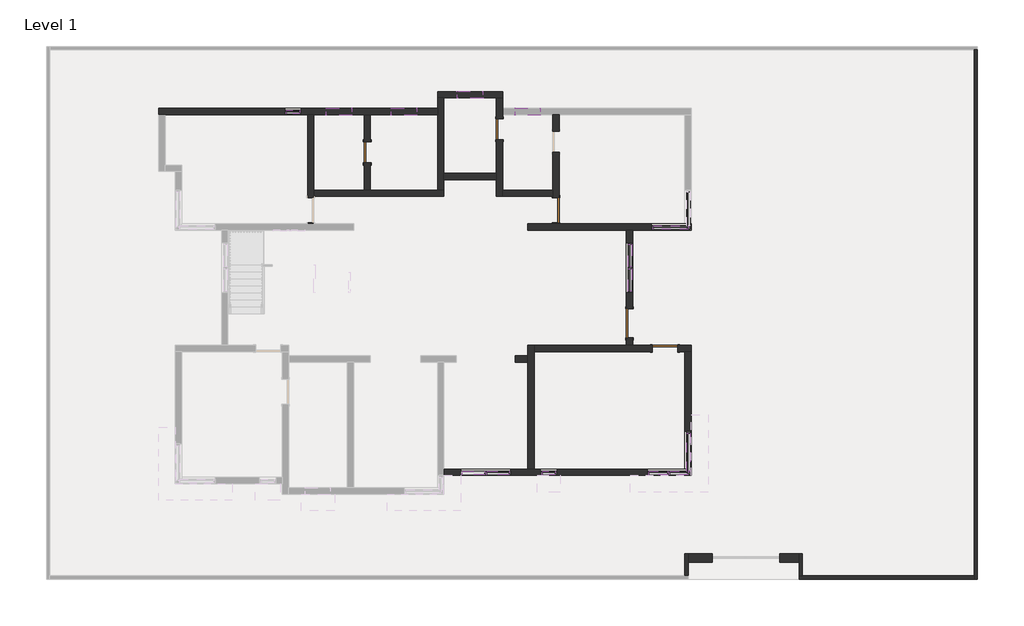
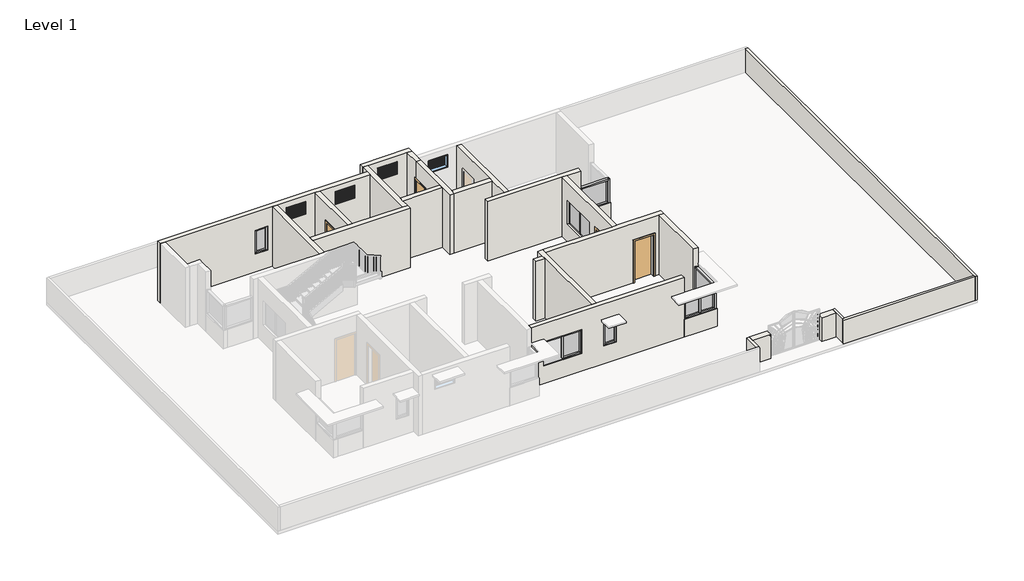
# One storey, part 2 of 9: 37 members, 27 walls, 9 plates, 5 doors, 4 windows.
"""IFC4 building model written with IfcOpenShell, lengths in millimetres."""

from ifc_helpers import new_model, si_unit, frame, origin, origin_with_axes, place, context, project, spatial, polyline, outline, extrude, faceted_brep, transform, mapped, element, save
from components import door_bb98abfd, single_flush_door_3_0ca8825f, door_0848dd25, member_75074519, member_5783932f, member_49503176, member_e1cf819f, member_6e28d7e1, member_2b49869a, member_c17f1be2, member_8d24a278, member_86d06fe4, system_panel_glazed_87944ff9, system_panel_glazed_e0df8542, system_panel_glazed_927b5fc9, system_panel_glazed_d6173012, system_panel_glazed_7cebc396, system_panel_glazed_1bcf12e0, window_a18e4be4

model = new_model("IFC4")

# Units and contexts
model_context = context("Model", 3, world=origin())
ifc_project = project(units=[si_unit("LENGTHUNIT", "METRE", prefix="MILLI")], contexts=[model_context])

# Site, building, storey
site = spatial("IfcSite", under=ifc_project)
building = spatial("IfcBuilding", under=site)
storey = spatial("IfcBuildingStorey", under=building, Name="Level 1", Elevation=0.0)

# Doors
placement = place(None, origin())
door_shape = door_bb98abfd(model_context)
element("IfcDoor", 1, ObjectType="Single-Flush : door 2'6\"", at=placement, inside=storey, context=model_context, shape_type="MappedRepresentation", body=[
    mapped(door_shape, transform((-35934.4146233, 18282.7624892, 0.0), x_axis=(0.0, 1.0, 0.0), y_axis=(-1.0, 0.0, 0.0), z_axis=(0.0, 0.0, 1.0))),
])
element("IfcDoor", 2, ObjectType="Single-Flush : door 2'6\"", at=placement, inside=storey, context=model_context, shape_type="MappedRepresentation", body=[
    mapped(door_shape, transform((-31133.8146233, 19120.9624892, 0.0), x_axis=(0.0, 1.0, 0.0), y_axis=(-1.0, 0.0, 0.0), z_axis=(0.0, 0.0, 1.0))),
])
single_flush_door_3_shape = single_flush_door_3_0ca8825f(model_context)
element("IfcDoor", 3, ObjectType="Single-Flush : door 3'", at=placement, inside=storey, context=model_context, shape_type="MappedRepresentation", body=[
    mapped(single_flush_door_3_shape, transform((-25114.0146233, 11158.0624892, 0.0), x_axis=(1.0, 0.0, 0.0), y_axis=(0.0, 1.0, 0.0), z_axis=(0.0, 0.0, 1.0))),
])
element("IfcDoor", 4, ObjectType="Single-Flush : door 3'", at=placement, inside=storey, context=model_context, shape_type="MappedRepresentation", body=[
    mapped(single_flush_door_3_shape, transform((-29076.4146233, 16187.2624892, 0.0), x_axis=(0.0, -1.0, 0.0), y_axis=(1.0, 0.0, 0.0), z_axis=(0.0, 0.0, 1.0))),
])
door_2_shape = door_0848dd25(model_context)
element("IfcDoor", 5, ObjectType="Single-Flush : door 3'6\"", at=placement, inside=storey, context=model_context, shape_type="MappedRepresentation", body=[
    mapped(door_2_shape, transform((-26409.4146233, 12072.4624892, 0.0), x_axis=(0.0, -1.0, 0.0), y_axis=(1.0, 0.0, 0.0), z_axis=(0.0, 0.0, 1.0))),
])

# Members
member_shape = member_75074519(model_context)
element("IfcMember", 6, ObjectType="Rectangular Mullion : 2.5\" x 5\" rectangular", at=placement, inside=storey, context=model_context, shape_type="MappedRepresentation", body=[
    mapped(member_shape, transform((-24199.6146233, 15552.2624892, 914.4), x_axis=(1.0, 0.0, 0.0), y_axis=(0.0, -1.0, 0.0), z_axis=(0.0, 0.0, -1.0))),
])
element("IfcMember", 7, ObjectType="Rectangular Mullion : 2.5\" x 5\" rectangular", at=placement, inside=storey, context=model_context, shape_type="MappedRepresentation", body=[
    mapped(member_shape, transform((-24199.6146233, 6636.8624892, 914.4), x_axis=(1.0, 0.0, 0.0), y_axis=(0.0, -1.0, 0.0), z_axis=(0.0, 0.0, -1.0))),
])
element("IfcMember", 8, ObjectType="Rectangular Mullion : 2.5\" x 5\" rectangular", at=placement, inside=storey, context=model_context, shape_type="MappedRepresentation", body=[
    mapped(member_shape, transform((-24263.1146233, 8148.1624892, 914.4), x_axis=(0.0, 1.0, 0.0), y_axis=(1.0, 0.0, 0.0), z_axis=(0.0, 0.0, -1.0))),
])
element("IfcMember", 9, ObjectType="Rectangular Mullion : 2.5\" x 5\" rectangular", at=placement, inside=storey, context=model_context, shape_type="MappedRepresentation", body=[
    mapped(member_shape, transform((-30714.7146233, 6636.8624892, 914.4), x_axis=(1.0, 0.0, 0.0), y_axis=(0.0, -1.0, 0.0), z_axis=(0.0, 0.0, -1.0))),
])
element("IfcMember", 10, ObjectType="Rectangular Mullion : 2.5\" x 5\" rectangular", at=placement, inside=storey, context=model_context, shape_type="MappedRepresentation", body=[
    mapped(member_shape, transform((-26383.9055559, 15005.5684528, 914.4), x_axis=(0.0, 1.0, 0.0), y_axis=(1.0, 0.0, 0.0), z_axis=(0.0, 0.0, -1.0))),
])
element("IfcMember", 11, ObjectType="Rectangular Mullion : 2.5\" x 5\" rectangular", at=placement, inside=storey, context=model_context, shape_type="MappedRepresentation", body=[
    mapped(member_shape, transform((-38334.7146233, 19743.2624892, 914.4), x_axis=(1.0, 0.0, 0.0), y_axis=(0.0, -1.0, 0.0), z_axis=(0.0, 0.0, -1.0))),
])
element("IfcMember", 12, ObjectType="Rectangular Mullion : 2.5\" x 5\" rectangular", at=placement, inside=storey, context=model_context, shape_type="MappedRepresentation", body=[
    mapped(member_shape, transform((-29038.3146233, 6636.8624892, 914.4), x_axis=(1.0, 0.0, 0.0), y_axis=(0.0, -1.0, 0.0), z_axis=(0.0, 0.0, -1.0))),
])
element("IfcMember", 13, ObjectType="Rectangular Mullion : 2.5\" x 5\" rectangular", at=placement, inside=storey, context=model_context, shape_type="MappedRepresentation", body=[
    mapped(member_shape, transform((-25609.3146233, 15552.2624892, 2133.6), x_axis=(-1.0, 0.0, 0.0), y_axis=(0.0, -1.0, 0.0), z_axis=(0.0, 0.0, 1.0))),
])
element("IfcMember", 14, ObjectType="Rectangular Mullion : 2.5\" x 5\" rectangular", at=placement, inside=storey, context=model_context, shape_type="MappedRepresentation", body=[
    mapped(member_shape, transform((-24263.1146233, 15552.2624892, 2133.6), x_axis=(0.0, -1.0, 0.0), y_axis=(1.0, 0.0, 0.0), z_axis=(0.0, 0.0, 1.0))),
])
element("IfcMember", 15, ObjectType="Rectangular Mullion : 2.5\" x 5\" rectangular", at=placement, inside=storey, context=model_context, shape_type="MappedRepresentation", body=[
    mapped(member_shape, transform((-25761.7146233, 6636.8624892, 2133.6), x_axis=(-1.0, 0.0, 0.0), y_axis=(0.0, -1.0, 0.0), z_axis=(0.0, 0.0, 1.0))),
])
element("IfcMember", 16, ObjectType="Rectangular Mullion : 2.5\" x 5\" rectangular", at=placement, inside=storey, context=model_context, shape_type="MappedRepresentation", body=[
    mapped(member_shape, transform((-24263.1146233, 6636.8624892, 2133.6), x_axis=(0.0, -1.0, 0.0), y_axis=(1.0, 0.0, 0.0), z_axis=(0.0, 0.0, 1.0))),
])
element("IfcMember", 17, ObjectType="Rectangular Mullion : 2.5\" x 5\" rectangular", at=placement, inside=storey, context=model_context, shape_type="MappedRepresentation", body=[
    mapped(member_shape, transform((-26383.9055559, 13177.3624892, 2133.6), x_axis=(0.0, -1.0, 0.0), y_axis=(1.0, 0.0, 0.0), z_axis=(0.0, 0.0, 1.0))),
])
element("IfcMember", 18, ObjectType="Rectangular Mullion : 2.5\" x 5\" rectangular", at=placement, inside=storey, context=model_context, shape_type="MappedRepresentation", body=[
    mapped(member_shape, transform((-38944.3146233, 19743.2624892, 2133.6), x_axis=(-1.0, 0.0, 0.0), y_axis=(0.0, -1.0, 0.0), z_axis=(0.0, 0.0, 1.0))),
])
element("IfcMember", 19, ObjectType="Rectangular Mullion : 2.5\" x 5\" rectangular", at=placement, inside=storey, context=model_context, shape_type="MappedRepresentation", body=[
    mapped(member_shape, transform((-29647.9146233, 6636.8624892, 2133.6), x_axis=(-1.0, 0.0, 0.0), y_axis=(0.0, -1.0, 0.0), z_axis=(0.0, 0.0, 1.0))),
])
member_2_shape = member_5783932f(model_context)
element("IfcMember", 20, ObjectType="Rectangular Mullion : 2.5\" x 5\" rectangular", at=placement, inside=storey, context=model_context, shape_type="MappedRepresentation", body=[
    mapped(member_2_shape, transform((-24263.1146233, 15552.2624892, 2133.6), x_axis=(0.0, 0.0, 1.0), y_axis=(0.0, -1.0, 0.0), z_axis=(1.0, 0.0, 0.0))),
])
element("IfcMember", 21, ObjectType="Rectangular Mullion : 2.5\" x 5\" rectangular", at=placement, inside=storey, context=model_context, shape_type="MappedRepresentation", body=[
    mapped(member_2_shape, transform((-25545.8146233, 15552.2624892, 914.4), x_axis=(0.0, 0.0, -1.0), y_axis=(0.0, -1.0, 0.0), z_axis=(-1.0, 0.0, 0.0))),
])
member_3_shape = member_49503176(model_context)
element("IfcMember", 22, ObjectType="Rectangular Mullion : 2.5\" x 5\" rectangular", at=placement, inside=storey, context=model_context, shape_type="MappedRepresentation", body=[
    mapped(member_3_shape, transform((-24263.1146233, 15615.7624892, 914.4), x_axis=(0.0, 0.0, -1.0), y_axis=(1.0, 0.0, 0.0), z_axis=(0.0, -1.0, 0.0))),
])
member_4_shape = member_e1cf819f(model_context)
element("IfcMember", 23, ObjectType="Rectangular Mullion : 2.5\" x 5\" rectangular", at=placement, inside=storey, context=model_context, shape_type="MappedRepresentation", body=[
    mapped(member_4_shape, transform((-24263.1146233, 8084.6624892, 2133.6), x_axis=(0.0, 0.0, 1.0), y_axis=(1.0, 0.0, 0.0), z_axis=(0.0, 1.0, 0.0))),
])
element("IfcMember", 24, ObjectType="Rectangular Mullion : 2.5\" x 5\" rectangular", at=placement, inside=storey, context=model_context, shape_type="MappedRepresentation", body=[
    mapped(member_4_shape, transform((-24263.1146233, 6700.3624892, 914.4), x_axis=(0.0, 0.0, -1.0), y_axis=(1.0, 0.0, 0.0), z_axis=(0.0, -1.0, 0.0))),
])
member_5_shape = member_6e28d7e1(model_context)
element("IfcMember", 25, ObjectType="Rectangular Mullion : 2.5\" x 5\" rectangular", at=placement, inside=storey, context=model_context, shape_type="MappedRepresentation", body=[
    mapped(member_5_shape, transform((-24263.1146233, 6636.8624892, 2133.6), x_axis=(0.0, 0.0, 1.0), y_axis=(0.0, -1.0, 0.0), z_axis=(1.0, 0.0, 0.0))),
])
element("IfcMember", 26, ObjectType="Rectangular Mullion : 2.5\" x 5\" rectangular", at=placement, inside=storey, context=model_context, shape_type="MappedRepresentation", body=[
    mapped(member_5_shape, transform((-25012.4146233, 6636.8624892, 2133.6), x_axis=(0.0, 0.0, 1.0), y_axis=(0.0, -1.0, 0.0), z_axis=(1.0, 0.0, 0.0))),
])
element("IfcMember", 27, ObjectType="Rectangular Mullion : 2.5\" x 5\" rectangular", at=placement, inside=storey, context=model_context, shape_type="MappedRepresentation", body=[
    mapped(member_5_shape, transform((-25698.2146233, 6636.8624892, 914.4), x_axis=(0.0, 0.0, -1.0), y_axis=(0.0, -1.0, 0.0), z_axis=(-1.0, 0.0, 0.0))),
])
element("IfcMember", 28, ObjectType="Rectangular Mullion : 2.5\" x 5\" rectangular", at=placement, inside=storey, context=model_context, shape_type="MappedRepresentation", body=[
    mapped(member_5_shape, transform((-24948.9146233, 6636.8624892, 914.4), x_axis=(0.0, 0.0, -1.0), y_axis=(0.0, -1.0, 0.0), z_axis=(-1.0, 0.0, 0.0))),
])
member_6_shape = member_2b49869a(model_context)
element("IfcMember", 29, ObjectType="Rectangular Mullion : 2.5\" x 5\" rectangular", at=placement, inside=storey, context=model_context, shape_type="MappedRepresentation", body=[
    mapped(member_6_shape, transform((-24980.6646233, 6636.8624892, 914.4), x_axis=(1.0, 0.0, 0.0), y_axis=(0.0, -1.0, 0.0), z_axis=(0.0, 0.0, -1.0))),
])
element("IfcMember", 30, ObjectType="Rectangular Mullion : 2.5\" x 5\" rectangular", at=placement, inside=storey, context=model_context, shape_type="MappedRepresentation", body=[
    mapped(member_6_shape, transform((-31629.1146233, 6636.8624892, 914.4), x_axis=(1.0, 0.0, 0.0), y_axis=(0.0, -1.0, 0.0), z_axis=(0.0, 0.0, -1.0))),
])
element("IfcMember", 31, ObjectType="Rectangular Mullion : 2.5\" x 5\" rectangular", at=placement, inside=storey, context=model_context, shape_type="MappedRepresentation", body=[
    mapped(member_6_shape, transform((-26383.9055559, 14091.465471, 914.4), x_axis=(0.0, 1.0, 0.0), y_axis=(1.0, 0.0, 0.0), z_axis=(0.0, 0.0, -1.0))),
])
member_7_shape = member_c17f1be2(model_context)
element("IfcMember", 32, ObjectType="Rectangular Mullion : 2.5\" x 5\" rectangular", at=placement, inside=storey, context=model_context, shape_type="MappedRepresentation", body=[
    mapped(member_7_shape, transform((-30778.2146233, 6636.8624892, 2133.6), x_axis=(0.0, 0.0, 1.0), y_axis=(0.0, -1.0, 0.0), z_axis=(1.0, 0.0, 0.0))),
])
element("IfcMember", 33, ObjectType="Rectangular Mullion : 2.5\" x 5\" rectangular", at=placement, inside=storey, context=model_context, shape_type="MappedRepresentation", body=[
    mapped(member_7_shape, transform((-31660.8646233, 6636.8624892, 2133.6), x_axis=(0.0, 0.0, 1.0), y_axis=(0.0, -1.0, 0.0), z_axis=(1.0, 0.0, 0.0))),
])
element("IfcMember", 34, ObjectType="Rectangular Mullion : 2.5\" x 5\" rectangular", at=placement, inside=storey, context=model_context, shape_type="MappedRepresentation", body=[
    mapped(member_7_shape, transform((-31597.3646233, 6636.8624892, 914.4), x_axis=(0.0, 0.0, -1.0), y_axis=(0.0, -1.0, 0.0), z_axis=(-1.0, 0.0, 0.0))),
])
member_8_shape = member_8d24a278(model_context)
element("IfcMember", 35, ObjectType="Rectangular Mullion : 2.5\" x 5\" rectangular", at=placement, inside=storey, context=model_context, shape_type="MappedRepresentation", body=[
    mapped(member_8_shape, transform((-26383.9055559, 14942.0684528, 2133.6), x_axis=(0.0, 0.0, 1.0), y_axis=(1.0, 0.0, 0.0), z_axis=(0.0, 1.0, 0.0))),
])
element("IfcMember", 36, ObjectType="Rectangular Mullion : 2.5\" x 5\" rectangular", at=placement, inside=storey, context=model_context, shape_type="MappedRepresentation", body=[
    mapped(member_8_shape, transform((-26383.9055559, 14059.715471, 2133.6), x_axis=(0.0, 0.0, 1.0), y_axis=(1.0, 0.0, 0.0), z_axis=(0.0, 1.0, 0.0))),
])
element("IfcMember", 37, ObjectType="Rectangular Mullion : 2.5\" x 5\" rectangular", at=placement, inside=storey, context=model_context, shape_type="MappedRepresentation", body=[
    mapped(member_8_shape, transform((-26383.9055559, 13240.8624892, 914.4), x_axis=(0.0, 0.0, -1.0), y_axis=(1.0, 0.0, 0.0), z_axis=(0.0, -1.0, 0.0))),
])
element("IfcMember", 38, ObjectType="Rectangular Mullion : 2.5\" x 5\" rectangular", at=placement, inside=storey, context=model_context, shape_type="MappedRepresentation", body=[
    mapped(member_8_shape, transform((-26383.9055559, 14123.215471, 914.4), x_axis=(0.0, 0.0, -1.0), y_axis=(1.0, 0.0, 0.0), z_axis=(0.0, -1.0, 0.0))),
])
member_9_shape = member_86d06fe4(model_context)
element("IfcMember", 39, ObjectType="Rectangular Mullion : 2.5\" x 5\" rectangular", at=placement, inside=storey, context=model_context, shape_type="MappedRepresentation", body=[
    mapped(member_9_shape, transform((-38398.2146233, 19743.2624892, 2133.6), x_axis=(0.0, 0.0, 1.0), y_axis=(0.0, -1.0, 0.0), z_axis=(1.0, 0.0, 0.0))),
])
element("IfcMember", 40, ObjectType="Rectangular Mullion : 2.5\" x 5\" rectangular", at=placement, inside=storey, context=model_context, shape_type="MappedRepresentation", body=[
    mapped(member_9_shape, transform((-29101.8146233, 6636.8624892, 2133.6), x_axis=(0.0, 0.0, 1.0), y_axis=(0.0, -1.0, 0.0), z_axis=(1.0, 0.0, 0.0))),
])
element("IfcMember", 41, ObjectType="Rectangular Mullion : 2.5\" x 5\" rectangular", at=placement, inside=storey, context=model_context, shape_type="MappedRepresentation", body=[
    mapped(member_9_shape, transform((-38880.8146233, 19743.2624892, 914.4), x_axis=(0.0, 0.0, -1.0), y_axis=(0.0, -1.0, 0.0), z_axis=(-1.0, 0.0, 0.0))),
])
element("IfcMember", 42, ObjectType="Rectangular Mullion : 2.5\" x 5\" rectangular", at=placement, inside=storey, context=model_context, shape_type="MappedRepresentation", body=[
    mapped(member_9_shape, transform((-29584.4146233, 6636.8624892, 914.4), x_axis=(0.0, 0.0, -1.0), y_axis=(0.0, -1.0, 0.0), z_axis=(-1.0, 0.0, 0.0))),
])

# Plates
system_panel_glazed_shape = system_panel_glazed_87944ff9(model_context)
element("IfcPlate", 43, ObjectType="System Panel : Glazed", at=placement, inside=storey, context=model_context, shape_type="MappedRepresentation", body=[
    mapped(system_panel_glazed_shape, transform((-24904.4646233, 15552.2624892, 977.9), x_axis=(1.0, 0.0, 0.0), y_axis=(0.0, 1.0, 0.0), z_axis=(0.0, 0.0, 1.0))),
])
system_panel_glazed_2_shape = system_panel_glazed_e0df8542(model_context)
element("IfcPlate", 44, ObjectType="System Panel : Glazed", at=placement, inside=storey, context=model_context, shape_type="MappedRepresentation", body=[
    mapped(system_panel_glazed_2_shape, transform((-24263.1146233, 7392.5124892, 977.9), x_axis=(0.0, 1.0, 0.0), y_axis=(-1.0, 0.0, 0.0), z_axis=(0.0, 0.0, 1.0))),
])
system_panel_glazed_3_shape = system_panel_glazed_927b5fc9(model_context)
element("IfcPlate", 45, ObjectType="System Panel : Glazed", at=placement, inside=storey, context=model_context, shape_type="MappedRepresentation", body=[
    mapped(system_panel_glazed_3_shape, transform((-25355.3146233, 6636.8624892, 977.9), x_axis=(1.0, 0.0, 0.0), y_axis=(0.0, 1.0, 0.0), z_axis=(0.0, 0.0, 1.0))),
])
element("IfcPlate", 46, ObjectType="System Panel : Glazed", at=placement, inside=storey, context=model_context, shape_type="MappedRepresentation", body=[
    mapped(system_panel_glazed_3_shape, transform((-24606.0146233, 6636.8624892, 977.9), x_axis=(1.0, 0.0, 0.0), y_axis=(0.0, 1.0, 0.0), z_axis=(0.0, 0.0, 1.0))),
])
system_panel_glazed_4_shape = system_panel_glazed_d6173012(model_context)
element("IfcPlate", 47, ObjectType="System Panel : Glazed", at=placement, inside=storey, context=model_context, shape_type="MappedRepresentation", body=[
    mapped(system_panel_glazed_4_shape, transform((-31187.7896233, 6636.8624892, 977.9), x_axis=(1.0, 0.0, 0.0), y_axis=(0.0, 1.0, 0.0), z_axis=(0.0, 0.0, 1.0))),
])
system_panel_glazed_5_shape = system_panel_glazed_7cebc396(model_context)
element("IfcPlate", 48, ObjectType="System Panel : Glazed", at=placement, inside=storey, context=model_context, shape_type="MappedRepresentation", body=[
    mapped(system_panel_glazed_5_shape, transform((-26383.9055559, 13650.2889801, 977.9), x_axis=(0.0, 1.0, 0.0), y_axis=(-1.0, 0.0, 0.0), z_axis=(0.0, 0.0, 1.0))),
])
element("IfcPlate", 49, ObjectType="System Panel : Glazed", at=placement, inside=storey, context=model_context, shape_type="MappedRepresentation", body=[
    mapped(system_panel_glazed_5_shape, transform((-26383.9055559, 14532.6419619, 977.9), x_axis=(0.0, 1.0, 0.0), y_axis=(-1.0, 0.0, 0.0), z_axis=(0.0, 0.0, 1.0))),
])
system_panel_glazed_6_shape = system_panel_glazed_1bcf12e0(model_context)
element("IfcPlate", 50, ObjectType="System Panel : Glazed", at=placement, inside=storey, context=model_context, shape_type="MappedRepresentation", body=[
    mapped(system_panel_glazed_6_shape, transform((-38639.5146233, 19743.2624892, 977.9), x_axis=(1.0, 0.0, 0.0), y_axis=(0.0, 1.0, 0.0), z_axis=(0.0, 0.0, 1.0))),
])
element("IfcPlate", 51, ObjectType="System Panel : Glazed", at=placement, inside=storey, context=model_context, shape_type="MappedRepresentation", body=[
    mapped(system_panel_glazed_6_shape, transform((-29343.1146233, 6636.8624892, 977.9), x_axis=(1.0, 0.0, 0.0), y_axis=(0.0, 1.0, 0.0), z_axis=(0.0, 0.0, 1.0))),
])

# Walls
element("IfcWall", 52, at=placement, inside=storey, context=model_context, shape_type="Brep", body=[
    faceted_brep([(-13874.5146233, 22016.5624892, 0.0), (-13874.5146233, 2890.3624892, 0.0), (-13874.5146233, 2776.0624892, 0.0), (-13874.5146233, 2776.0624892, 1219.2), (-13874.5146233, 2890.3624892, 1219.2), (-13874.5146233, 22016.5624892, 1219.2), (-13760.2146233, 22016.5624892, 0.0), (-13760.2146233, 22016.5624892, 1219.2), (-13760.2146233, 2776.0624892, 1219.2), (-13760.2146233, 2776.0624892, 0.0)], [[[0, 1, 2, 3, 4, 5]], [[6, 7, 8, 9]], [[2, 1, 0, 6, 9]], [[5, 4, 3, 8, 7]], [[0, 5, 7, 6]], [[3, 2, 9, 8]]]),
])
element("IfcWall", 53, at=placement, inside=storey, context=model_context, shape_type="Brep", body=[
    faceted_brep([(-13874.5146233, 2890.3624892, 0.0), (-20122.9146233, 2890.3624892, 0.0), (-20237.2146233, 2890.3624892, 0.0), (-20237.2146233, 2890.3624892, 1219.2), (-20122.9146233, 2890.3624892, 1219.2), (-13874.5146233, 2890.3624892, 1219.2), (-13874.5146233, 2776.0624892, 0.0), (-13874.5146233, 2776.0624892, 1219.2), (-20237.2146233, 2776.0624892, 1219.2), (-20237.2146233, 2776.0624892, 0.0)], [[[0, 1, 2, 3, 4, 5]], [[6, 7, 8, 9]], [[2, 1, 0, 6, 9]], [[5, 4, 3, 8, 7]], [[0, 5, 7, 6]], [[3, 2, 9, 8]]]),
])
element("IfcWall", 54, at=placement, inside=storey, context=model_context, shape_type="Brep", body=[
    faceted_brep([(-20122.9146233, 2890.3624892, 0.0), (-20122.9146233, 3690.4624892, 0.0), (-20122.9146233, 3690.4624892, 1219.2), (-20122.9146233, 2890.3624892, 1219.2), (-20237.2146233, 2890.3624892, 0.0), (-20237.2146233, 2890.3624892, 1219.2), (-20237.2146233, 3385.6624892, 1219.2), (-20237.2146233, 3690.4624892, 1219.2), (-20237.2146233, 3690.4624892, 0.0), (-20237.2146233, 3385.6624892, 0.0)], [[[0, 1, 2, 3]], [[4, 5, 6, 7, 8, 9]], [[1, 0, 4, 9, 8]], [[3, 2, 7, 6, 5]], [[0, 3, 5, 4]], [[2, 1, 8, 7]]]),
])
element("IfcWall", 55, at=placement, inside=storey, context=model_context, shape_type="Brep", body=[
    faceted_brep([(-24275.8146233, 2890.3624892, 0.0), (-24275.8146233, 3385.6624892, 0.0), (-24275.8146233, 3690.4624892, 0.0), (-24275.8146233, 3690.4624892, 1219.2), (-24275.8146233, 3385.6624892, 1219.2), (-24275.8146233, 2890.3624892, 1219.2), (-24390.1146233, 2890.3624892, 0.0), (-24390.1146233, 2890.3624892, 1219.2), (-24390.1146233, 3690.4624892, 1219.2), (-24390.1146233, 3690.4624892, 0.0)], [[[0, 1, 2, 3, 4, 5]], [[6, 7, 8, 9]], [[2, 1, 0, 6, 9]], [[5, 4, 3, 8, 7]], [[0, 5, 7, 6]], [[3, 2, 9, 8]]]),
])
element("IfcWall", 56, ObjectType="WALL 9\"", at=placement, inside=storey, context=model_context, shape_type="Brep", body=[
    faceted_brep([(-43516.3146233, 19654.3624892, 0.0), (-43287.7146233, 19654.3624892, 0.0), (-38106.1146233, 19654.3624892, 0.0), (-37877.5146233, 19654.3624892, 0.0), (-36048.7146233, 19654.3624892, 0.0), (-35820.1146233, 19654.3624892, 0.0), (-33381.7146233, 19654.3624892, 0.0), (-33381.7146233, 19654.3624892, 3048.0), (-35820.1146233, 19654.3624892, 3048.0), (-36048.7146233, 19654.3624892, 3048.0), (-37877.5146233, 19654.3624892, 3048.0), (-38106.1146233, 19654.3624892, 3048.0), (-43287.7146233, 19654.3624892, 3048.0), (-43516.3146233, 19654.3624892, 3048.0), (-38944.3146233, 19654.3624892, 914.4), (-38944.3146233, 19654.3624892, 2133.6), (-38334.7146233, 19654.3624892, 2133.6), (-38334.7146233, 19654.3624892, 914.4), (-36505.9146233, 19654.3624892, 2743.2), (-36505.9146233, 19654.3624892, 2133.6), (-37420.3146233, 19654.3624892, 2133.6), (-37420.3146233, 19654.3624892, 2743.2), (-34143.7146233, 19654.3624892, 2743.2), (-34143.7146233, 19654.3624892, 2133.6), (-35058.1146233, 19654.3624892, 2133.6), (-35058.1146233, 19654.3624892, 2743.2), (-33381.7146233, 19882.9624892, 0.0), (-43516.3146233, 19882.9624892, 0.0), (-43516.3146233, 19882.9624892, 3048.0), (-33381.7146233, 19882.9624892, 3048.0), (-38944.3146233, 19882.9624892, 2133.6), (-38944.3146233, 19882.9624892, 914.4), (-38334.7146233, 19882.9624892, 914.4), (-38334.7146233, 19882.9624892, 2133.6), (-36505.9146233, 19882.9624892, 2743.2), (-37420.3146233, 19882.9624892, 2743.2), (-37420.3146233, 19882.9624892, 2133.6), (-36505.9146233, 19882.9624892, 2133.6), (-34143.7146233, 19882.9624892, 2743.2), (-35058.1146233, 19882.9624892, 2743.2), (-35058.1146233, 19882.9624892, 2133.6), (-34143.7146233, 19882.9624892, 2133.6)], [[[0, 1, 2, 3, 4, 5, 6, 7, 8, 9, 10, 11, 12, 13], [14, 15, 16, 17], [18, 19, 20, 21], [22, 23, 24, 25]], [[26, 27, 28, 29], [30, 31, 32, 33], [34, 35, 36, 37], [38, 39, 40, 41]], [[6, 5, 4, 3, 2, 1, 0, 27, 26]], [[13, 12, 11, 10, 9, 8, 7, 29, 28]], [[0, 13, 28, 27]], [[7, 6, 26, 29]], [[14, 31, 30, 15]], [[15, 30, 33, 16]], [[16, 33, 32, 17]], [[31, 14, 17, 32]], [[19, 18, 34, 37]], [[20, 19, 37, 36]], [[21, 20, 36, 35]], [[18, 21, 35, 34]], [[23, 22, 38, 41]], [[24, 23, 41, 40]], [[25, 24, 40, 39]], [[22, 25, 39, 38]]]),
])
element("IfcWall", 57, ObjectType="WALL 9\"", at=placement, inside=storey, context=model_context, shape_type="Brep", body=[
    faceted_brep([(-33381.7146233, 20263.9624892, 0.0), (-33153.1146233, 20263.9624892, 0.0), (-31248.1146233, 20263.9624892, 0.0), (-31019.5146233, 20263.9624892, 0.0), (-31019.5146233, 20263.9624892, 3048.0), (-31248.1146233, 20263.9624892, 3048.0), (-33153.1146233, 20263.9624892, 3048.0), (-33381.7146233, 20263.9624892, 3048.0), (-31743.4146233, 20263.9624892, 2743.2), (-31743.4146233, 20263.9624892, 2133.6), (-32657.8146233, 20263.9624892, 2133.6), (-32657.8146233, 20263.9624892, 2743.2), (-33381.7146233, 20492.5624892, 0.0), (-33381.7146233, 20492.5624892, 3048.0), (-31019.5146233, 20492.5624892, 3048.0), (-31019.5146233, 20492.5624892, 0.0), (-31743.4146233, 20492.5624892, 2743.2), (-32657.8146233, 20492.5624892, 2743.2), (-32657.8146233, 20492.5624892, 2133.6), (-31743.4146233, 20492.5624892, 2133.6)], [[[0, 1, 2, 3, 4, 5, 6, 7], [8, 9, 10, 11]], [[12, 13, 14, 15], [16, 17, 18, 19]], [[3, 2, 1, 0, 12, 15]], [[7, 6, 5, 4, 14, 13]], [[4, 3, 15, 14]], [[0, 7, 13, 12]], [[9, 8, 16, 19]], [[10, 9, 19, 18]], [[11, 10, 18, 17]], [[8, 11, 17, 16]]]),
])
element("IfcWall", 58, ObjectType="WALL 9\"", at=placement, inside=storey, context=model_context, shape_type="Brep", body=[
    faceted_brep([(-31248.1146233, 20263.9624892, 0.0), (-31248.1146233, 19501.9624892, 0.0), (-31248.1146233, 19501.9624892, 2133.6), (-31248.1146233, 19501.9624892, 3048.0), (-31248.1146233, 20263.9624892, 3048.0), (-31019.5146233, 20263.9624892, 0.0), (-31019.5146233, 20263.9624892, 3048.0), (-31019.5146233, 19882.9624892, 3048.0), (-31019.5146233, 19654.3624892, 3048.0), (-31019.5146233, 19501.9624892, 3048.0), (-31019.5146233, 19501.9624892, 2133.6), (-31019.5146233, 19501.9624892, 0.0), (-31019.5146233, 19654.3624892, 0.0), (-31019.5146233, 19882.9624892, 0.0)], [[[0, 1, 2, 3, 4]], [[5, 6, 7, 8, 9, 10, 11, 12, 13]], [[1, 0, 5, 13, 12, 11]], [[3, 2, 1, 11, 10, 9]], [[4, 3, 9, 8, 7, 6]], [[0, 4, 6, 5]]]),
])
element("IfcWall", 59, ObjectType="WALL 9\" 2", at=placement, inside=storey, context=model_context, shape_type="Brep", body=[
    faceted_brep([(-33152.7428374, 6547.9624892, 0.0), (-25761.7146233, 6547.9624892, 0.0), (-25761.7146233, 6547.9624892, 914.4), (-25761.7146233, 6547.9624892, 2133.6), (-25761.7146233, 6547.9624892, 3048.0), (-33152.7428374, 6547.9624892, 3048.0), (-32543.5146233, 6547.9624892, 914.4), (-32543.5146233, 6547.9624892, 2133.6), (-30714.7146233, 6547.9624892, 2133.6), (-30714.7146233, 6547.9624892, 914.4), (-29647.9146233, 6547.9624892, 914.4), (-29647.9146233, 6547.9624892, 2133.6), (-29038.3146233, 6547.9624892, 2133.6), (-29038.3146233, 6547.9624892, 914.4), (-25761.7146233, 6776.5624892, 0.0), (-29876.5146233, 6776.5624892, 0.0), (-30105.1146233, 6776.5624892, 0.0), (-33152.7428374, 6776.5624892, 0.0), (-33152.7428374, 6776.5624892, 3048.0), (-30105.1146233, 6776.5624892, 3048.0), (-29876.5146233, 6776.5624892, 3048.0), (-25761.7146233, 6776.5624892, 3048.0), (-25761.7146233, 6776.5624892, 2133.6), (-25761.7146233, 6776.5624892, 914.4), (-32543.5146233, 6776.5624892, 2133.6), (-32543.5146233, 6776.5624892, 914.4), (-30714.7146233, 6776.5624892, 914.4), (-30714.7146233, 6776.5624892, 2133.6), (-29647.9146233, 6776.5624892, 2133.6), (-29647.9146233, 6776.5624892, 914.4), (-29038.3146233, 6776.5624892, 914.4), (-29038.3146233, 6776.5624892, 2133.6)], [[[0, 1, 2, 3, 4, 5], [6, 7, 8, 9], [10, 11, 12, 13]], [[14, 15, 16, 17, 18, 19, 20, 21, 22, 23], [24, 25, 26, 27], [28, 29, 30, 31]], [[1, 0, 17, 16, 15, 14]], [[5, 4, 21, 20, 19, 18]], [[5, 18, 17, 0]], [[1, 14, 23, 22, 21, 4, 3, 2]], [[6, 25, 24, 7]], [[7, 24, 27, 8]], [[8, 27, 26, 9]], [[25, 6, 9, 26]], [[10, 29, 28, 11]], [[11, 28, 31, 12]], [[12, 31, 30, 13]], [[29, 10, 13, 30]]]),
])
element("IfcWall", 60, ObjectType="WALL 9\" 2", at=placement, inside=storey, context=model_context, shape_type="Brep", body=[
    faceted_brep([(-29876.5146233, 6776.5624892, 0.0), (-29876.5146233, 11043.7624892, 0.0), (-29876.5146233, 11272.3624892, 0.0), (-29876.5146233, 11272.3624892, 3048.0), (-29876.5146233, 11043.7624892, 3048.0), (-29876.5146233, 6776.5624892, 3048.0), (-30105.1146233, 6776.5624892, 0.0), (-30105.1146233, 6776.5624892, 3048.0), (-30105.1146233, 10662.7624892, 3048.0), (-30105.1146233, 10891.3624892, 3048.0), (-30105.1146233, 11272.3624892, 3048.0), (-30105.1146233, 11272.3624892, 0.0), (-30105.1146233, 10891.3624892, 0.0), (-30105.1146233, 10662.7624892, 0.0)], [[[0, 1, 2, 3, 4, 5]], [[6, 7, 8, 9, 10, 11, 12, 13]], [[2, 1, 0, 6, 13, 12, 11]], [[5, 4, 3, 10, 9, 8, 7]], [[0, 5, 7, 6]], [[3, 2, 11, 10]]]),
])
element("IfcWall", 61, ObjectType="WALL 9\" 2", at=placement, inside=storey, context=model_context, shape_type="Brep", body=[
    faceted_brep([(-24656.8146233, 11043.7624892, 2133.6), (-24656.8146233, 11043.7624892, 0.0), (-24390.1146233, 11043.7624892, 0.0), (-24161.5146233, 11043.7624892, 0.0), (-24161.5146233, 11043.7624892, 3048.0), (-24390.1146233, 11043.7624892, 3048.0), (-29876.5146233, 11043.7624892, 3048.0), (-29876.5146233, 11043.7624892, 0.0), (-25571.2146233, 11043.7624892, 0.0), (-25571.2146233, 11043.7624892, 2133.6), (-24161.5146233, 11272.3624892, 0.0), (-24656.8146233, 11272.3624892, 0.0), (-24656.8146233, 11272.3624892, 2133.6), (-25571.2146233, 11272.3624892, 2133.6), (-25571.2146233, 11272.3624892, 0.0), (-26295.1146233, 11272.3624892, 0.0), (-26523.7146233, 11272.3624892, 0.0), (-29876.5146233, 11272.3624892, 0.0), (-29876.5146233, 11272.3624892, 3048.0), (-26523.7146233, 11272.3624892, 3048.0), (-26295.1146233, 11272.3624892, 3048.0), (-24161.5146233, 11272.3624892, 3048.0)], [[[0, 1, 2, 3, 4, 5, 6, 7, 8, 9]], [[10, 11, 12, 13, 14, 15, 16, 17, 18, 19, 20, 21]], [[8, 7, 17, 16, 15, 14]], [[3, 2, 1, 11, 10]], [[6, 5, 4, 21, 20, 19, 18]], [[7, 6, 18, 17]], [[4, 3, 10, 21]], [[12, 11, 1, 0]], [[13, 12, 0, 9]], [[14, 13, 9, 8]]]),
])
element("IfcWall", 62, ObjectType="WALL 9\" 2", at=placement, inside=storey, context=model_context, shape_type="Brep", body=[
    faceted_brep([(-24390.1146233, 11043.7624892, 0.0), (-24390.1146233, 8148.1624892, 0.0), (-24390.1146233, 8148.1624892, 914.4), (-24390.1146233, 8148.1624892, 2133.6), (-24390.1146233, 8148.1624892, 3048.0), (-24390.1146233, 11043.7624892, 3048.0), (-24161.5146233, 11043.7624892, 0.0), (-24161.5146233, 11043.7624892, 3048.0), (-24161.5146233, 8148.1624892, 3048.0), (-24161.5146233, 8148.1624892, 2133.6), (-24161.5146233, 8148.1624892, 914.4), (-24161.5146233, 8148.1624892, 0.0)], [[[0, 1, 2, 3, 4, 5]], [[6, 7, 8, 9, 10, 11]], [[1, 0, 6, 11]], [[5, 4, 8, 7]], [[0, 5, 7, 6]], [[1, 11, 10, 9, 8, 4, 3, 2]]]),
])
element("IfcWall", 63, ObjectType="WALL 9\" 2", at=placement, inside=storey, context=model_context, shape_type="SweptSolid", body=[
    extrude(outline(polyline([(11539.0624892, 2133.6), (11539.0624892, 0.0), (11272.3624892, 0.0), (11272.3624892, 3048.0), (15463.3624892, 3048.0), (15463.3624892, 0.0), (12605.8624892, 0.0), (12605.8624892, 2133.6), (11539.0624892, 2133.6)]), holes=[polyline([(13177.3624892, 2133.6), (13177.3624892, 914.4), (15005.5684528, 914.4), (15005.5684528, 2133.6), (13177.3624892, 2133.6)])]), frame((-26523.7146233, 0.0, 0.0), z_axis=(1.0, 0.0, 0.0), x_axis=(0.0, 1.0, 0.0)), (0.0, 0.0, 1.0), 228.6),
])
element("IfcWall", 64, ObjectType="WALL 9\" 2", at=placement, inside=storey, context=model_context, shape_type="Brep", body=[
    faceted_brep([(-30105.1146233, 15463.3624892, 0.0), (-26523.7146233, 15463.3624892, 0.0), (-26295.1146233, 15463.3624892, 0.0), (-25609.3146233, 15463.3624892, 0.0), (-25609.3146233, 15463.3624892, 914.4), (-25609.3146233, 15463.3624892, 2133.6), (-25609.3146233, 15463.3624892, 3048.0), (-26295.1146233, 15463.3624892, 3048.0), (-26523.7146233, 15463.3624892, 3048.0), (-30105.1146233, 15463.3624892, 3048.0), (-30105.1146233, 15691.9624892, 0.0), (-30105.1146233, 15691.9624892, 3048.0), (-29190.7146233, 15691.9624892, 3048.0), (-28962.1146233, 15691.9624892, 3048.0), (-25609.3146233, 15691.9624892, 3048.0), (-25609.3146233, 15691.9624892, 2133.6), (-25609.3146233, 15691.9624892, 914.4), (-25609.3146233, 15691.9624892, 0.0), (-28962.1146233, 15691.9624892, 0.0), (-29190.7146233, 15691.9624892, 0.0)], [[[0, 1, 2, 3, 4, 5, 6, 7, 8, 9]], [[10, 11, 12, 13, 14, 15, 16, 17, 18, 19]], [[3, 2, 1, 0, 10, 19, 18, 17]], [[9, 8, 7, 6, 14, 13, 12, 11]], [[0, 9, 11, 10]], [[3, 17, 16, 15, 14, 6, 5, 4]]]),
])
element("IfcWall", 65, ObjectType="WALL 9\" 2", at=placement, inside=storey, context=model_context, shape_type="Brep", body=[
    faceted_brep([(-38106.1146233, 15725.5641869, 2133.6), (-38106.1146233, 15725.5641869, 0.0), (-38106.1146233, 15682.9658846, 0.0), (-38106.1146233, 15682.9658846, 3048.0), (-38106.1146233, 19654.3624892, 3048.0), (-38106.1146233, 19654.3624892, 0.0), (-38106.1146233, 16639.9641869, 0.0), (-38106.1146233, 16639.9641869, 2133.6), (-37877.5146233, 15682.9658846, 0.0), (-37877.5146233, 15725.5641869, 0.0), (-37877.5146233, 15725.5641869, 2133.6), (-37877.5146233, 16639.9641869, 2133.6), (-37877.5146233, 16639.9641869, 0.0), (-37877.5146233, 16682.5624892, 0.0), (-37877.5146233, 16911.1624892, 0.0), (-37877.5146233, 19654.3624892, 0.0), (-37877.5146233, 19654.3624892, 3048.0), (-37877.5146233, 16911.1624892, 3048.0), (-37877.5146233, 16682.5624892, 3048.0), (-37877.5146233, 15682.9658846, 3048.0)], [[[0, 1, 2, 3, 4, 5, 6, 7]], [[8, 9, 10, 11, 12, 13, 14, 15, 16, 17, 18, 19]], [[6, 5, 15, 14, 13, 12]], [[2, 1, 9, 8]], [[4, 3, 19, 18, 17, 16]], [[5, 4, 16, 15]], [[3, 2, 8, 19]], [[10, 9, 1, 0]], [[11, 10, 0, 7]], [[12, 11, 7, 6]]]),
])
element("IfcWall", 66, ObjectType="WALL 9\" 2", at=placement, inside=storey, context=model_context, shape_type="Brep", body=[
    faceted_brep([(-37877.5146233, 16682.5624892, 0.0), (-33153.1146233, 16682.5624892, 0.0), (-33153.1146233, 16682.5624892, 3048.0), (-37877.5146233, 16682.5624892, 3048.0), (-37877.5146233, 16911.1624892, 0.0), (-37877.5146233, 16911.1624892, 3048.0), (-36048.7146233, 16911.1624892, 3048.0), (-35820.1146233, 16911.1624892, 3048.0), (-33381.7146233, 16911.1624892, 3048.0), (-33153.1146233, 16911.1624892, 3048.0), (-33153.1146233, 16911.1624892, 0.0), (-33381.7146233, 16911.1624892, 0.0), (-35820.1146233, 16911.1624892, 0.0), (-36048.7146233, 16911.1624892, 0.0)], [[[0, 1, 2, 3]], [[4, 5, 6, 7, 8, 9, 10, 11, 12, 13]], [[1, 0, 4, 13, 12, 11, 10]], [[3, 2, 9, 8, 7, 6, 5]], [[2, 1, 10, 9]], [[0, 3, 5, 4]]]),
])
element("IfcWall", 67, ObjectType="WALL 9\" 2", at=placement, inside=storey, context=model_context, shape_type="SweptSolid", body=[
    extrude(outline(polyline([(19654.3624892, 0.0), (18663.7624892, 0.0), (18663.7624892, 2133.6), (17901.7624892, 2133.6), (17901.7624892, 0.0), (16911.1624892, 0.0), (16911.1624892, 3048.0), (19654.3624892, 3048.0), (19654.3624892, 0.0)])), frame((-36048.7146233, 0.0, 0.0), z_axis=(1.0, 0.0, 0.0), x_axis=(0.0, 1.0, 0.0)), (0.0, 0.0, 1.0), 228.6),
])
element("IfcWall", 68, ObjectType="WALL 9\" 2", at=placement, inside=storey, context=model_context, shape_type="Brep", body=[
    faceted_brep([(-33153.1146233, 16911.1624892, 0.0), (-33153.1146233, 17292.1624892, 0.0), (-33153.1146233, 17520.7624892, 0.0), (-33153.1146233, 20263.9624892, 0.0), (-33153.1146233, 20263.9624892, 3048.0), (-33153.1146233, 17520.7624892, 3048.0), (-33153.1146233, 17292.1624892, 3048.0), (-33153.1146233, 16911.1624892, 3048.0), (-33381.7146233, 16911.1624892, 0.0), (-33381.7146233, 16911.1624892, 3048.0), (-33381.7146233, 19654.3624892, 3048.0), (-33381.7146233, 19882.9624892, 3048.0), (-33381.7146233, 20263.9624892, 3048.0), (-33381.7146233, 20263.9624892, 0.0), (-33381.7146233, 19882.9624892, 0.0), (-33381.7146233, 19654.3624892, 0.0)], [[[0, 1, 2, 3, 4, 5, 6, 7]], [[8, 9, 10, 11, 12, 13, 14, 15]], [[3, 2, 1, 0, 8, 15, 14, 13]], [[7, 6, 5, 4, 12, 11, 10, 9]], [[4, 3, 13, 12]], [[0, 7, 9, 8]]]),
])
element("IfcWall", 69, ObjectType="WALL 9\" 2", at=placement, inside=storey, context=model_context, shape_type="SweptSolid", body=[
    extrude(outline(polyline([(-31248.1146233, 17292.1624892), (-33153.1146233, 17292.1624892), (-33153.1146233, 17520.7624892), (-31248.1146233, 17520.7624892), (-31248.1146233, 17292.1624892)])), origin_with_axes(), (0.0, 0.0, 1.0), 3048.0),
])
element("IfcWall", 70, ObjectType="WALL 9\" 2", at=placement, inside=storey, context=model_context, shape_type="Brep", body=[
    faceted_brep([(-31248.1146233, 16682.5624892, 3048.0), (-31248.1146233, 17292.1624892, 3048.0), (-31248.1146233, 17520.7624892, 3048.0), (-31248.1146233, 19501.9624892, 3048.0), (-31248.1146233, 19501.9624892, 2133.6), (-31248.1146233, 18739.9624892, 2133.6), (-31248.1146233, 18739.9624892, 0.0), (-31248.1146233, 17520.7624892, 0.0), (-31248.1146233, 17292.1624892, 0.0), (-31248.1146233, 16682.5624892, 0.0), (-31019.5146233, 19501.9624892, 3048.0), (-31019.5146233, 16911.1624892, 3048.0), (-31019.5146233, 16682.5624892, 3048.0), (-31019.5146233, 16682.5624892, 0.0), (-31019.5146233, 16911.1624892, 0.0), (-31019.5146233, 18739.9624892, 0.0), (-31019.5146233, 18739.9624892, 2133.6), (-31019.5146233, 19501.9624892, 2133.6)], [[[0, 1, 2, 3, 4, 5, 6, 7, 8, 9]], [[10, 11, 12, 13, 14, 15, 16, 17]], [[13, 9, 8, 7, 6, 15, 14]], [[3, 2, 1, 0, 12, 11, 10]], [[3, 10, 17, 4]], [[0, 9, 13, 12]], [[16, 5, 4, 17]], [[5, 16, 15, 6]]]),
])
element("IfcWall", 71, ObjectType="WALL 9\" 2", at=placement, inside=storey, context=model_context, shape_type="SweptSolid", body=[
    extrude(outline(polyline([(-29190.7146233, 16682.5624892), (-31019.5146233, 16682.5624892), (-31019.5146233, 16911.1624892), (-29190.7146233, 16911.1624892), (-29190.7146233, 16682.5624892)])), origin_with_axes(), (0.0, 0.0, 1.0), 3048.0),
])
element("IfcWall", 72, ObjectType="WALL 9\" 2", at=placement, inside=storey, context=model_context, shape_type="Brep", body=[
    faceted_brep([(-28962.1146233, 15691.9624892, 0.0), (-28962.1146233, 15730.0624892, 0.0), (-28962.1146233, 15730.0624892, 2133.6), (-28962.1146233, 16644.4624892, 2133.6), (-28962.1146233, 16644.4624892, 0.0), (-28962.1146233, 18295.4624892, 0.0), (-28962.1146233, 18295.4624892, 2133.6), (-28962.1146233, 19057.4624892, 2133.6), (-28962.1146233, 19057.4624892, 0.0), (-28962.1146233, 19654.3624892, 0.0), (-28962.1146233, 19654.3624892, 3048.0), (-28962.1146233, 15691.9624892, 3048.0), (-29190.7146233, 15730.0624892, 2133.6), (-29190.7146233, 15730.0624892, 0.0), (-29190.7146233, 15691.9624892, 0.0), (-29190.7146233, 15691.9624892, 3048.0), (-29190.7146233, 16682.5624892, 3048.0), (-29190.7146233, 16911.1624892, 3048.0), (-29190.7146233, 19654.3624892, 3048.0), (-29190.7146233, 19654.3624892, 0.0), (-29190.7146233, 19057.4624892, 0.0), (-29190.7146233, 19057.4624892, 2133.6), (-29190.7146233, 18295.4624892, 2133.6), (-29190.7146233, 18295.4624892, 0.0), (-29190.7146233, 16911.1624892, 0.0), (-29190.7146233, 16682.5624892, 0.0), (-29190.7146233, 16644.4624892, 0.0), (-29190.7146233, 16644.4624892, 2133.6)], [[[0, 1, 2, 3, 4, 5, 6, 7, 8, 9, 10, 11]], [[12, 13, 14, 15, 16, 17, 18, 19, 20, 21, 22, 23, 24, 25, 26, 27]], [[9, 8, 20, 19]], [[14, 13, 1, 0]], [[26, 25, 24, 23, 5, 4]], [[11, 10, 18, 17, 16, 15]], [[10, 9, 19, 18]], [[21, 20, 8, 7]], [[22, 21, 7, 6]], [[23, 22, 6, 5]], [[0, 11, 15, 14]], [[2, 1, 13, 12]], [[3, 2, 12, 27]], [[4, 3, 27, 26]]]),
])
element("IfcWall", 73, ObjectType="WALL 9\" 2", at=placement, inside=storey, context=model_context, shape_type="SweptSolid", body=[
    extrude(outline(polyline([(-30105.1146233, 10662.7624892), (-30562.3146233, 10662.7624892), (-30562.3146233, 10891.3624892), (-30105.1146233, 10891.3624892), (-30105.1146233, 10662.7624892)])), origin_with_axes(), (0.0, 0.0, 1.0), 3048.0),
])
element("IfcWall", 74, ObjectType="wall 1'", at=placement, inside=storey, context=model_context, shape_type="SweptSolid", body=[
    extrude(outline(polyline([(-20237.2146233, 3385.6624892), (-20945.2396233, 3385.6624892), (-20945.2396233, 3690.4624892), (-20237.2146233, 3690.4624892), (-20237.2146233, 3385.6624892)])), origin_with_axes(), (0.0, 0.0, 1.0), 1219.2),
])
element("IfcWall", 75, ObjectType="wall 1'", at=placement, inside=storey, context=model_context, shape_type="SweptSolid", body=[
    extrude(outline(polyline([(-24275.8146233, 3690.4624892), (-23402.6896233, 3690.4624892), (-23402.6896233, 3385.6624892), (-24275.8146233, 3385.6624892), (-24275.8146233, 3690.4624892)])), origin_with_axes(), (0.0, 0.0, 1.0), 1219.2),
])
element("IfcWall", 76, ObjectType="wall 3'", at=placement, inside=storey, context=model_context, shape_type="Brep", body=[
    faceted_brep([(-25609.3146233, 15463.3624892, 0.0), (-24161.5146233, 15463.3624892, 0.0), (-24161.5146233, 15463.3624892, 914.4), (-25609.3146233, 15463.3624892, 914.4), (-25609.3146233, 15691.9624892, 0.0), (-25609.3146233, 15691.9624892, 914.4), (-24390.1146233, 15691.9624892, 914.4), (-24161.5146233, 15691.9624892, 914.4), (-24161.5146233, 15691.9624892, 0.0), (-24390.1146233, 15691.9624892, 0.0)], [[[0, 1, 2, 3]], [[4, 5, 6, 7, 8, 9]], [[1, 0, 4, 9, 8]], [[3, 2, 7, 6, 5]], [[0, 3, 5, 4]], [[2, 1, 8, 7]]]),
])
element("IfcWall", 77, ObjectType="wall 3'", at=placement, inside=storey, context=model_context, shape_type="Brep", body=[
    faceted_brep([(-25761.7146233, 6547.9624892, 0.0), (-24161.5146233, 6547.9624892, 0.0), (-24161.5146233, 6547.9624892, 914.4), (-25761.7146233, 6547.9624892, 914.4), (-25761.7146233, 6776.5624892, 0.0), (-25761.7146233, 6776.5624892, 914.4), (-24390.1146233, 6776.5624892, 914.4), (-24161.5146233, 6776.5624892, 914.4), (-24161.5146233, 6776.5624892, 0.0), (-24390.1146233, 6776.5624892, 0.0)], [[[0, 1, 2, 3]], [[4, 5, 6, 7, 8, 9]], [[1, 0, 4, 9, 8]], [[3, 2, 7, 6, 5]], [[0, 3, 5, 4]], [[2, 1, 8, 7]]]),
])
element("IfcWall", 78, ObjectType="wall 3'", at=placement, inside=storey, context=model_context, shape_type="SweptSolid", body=[
    extrude(outline(polyline([(-24161.5146233, 8148.1624892), (-24161.5146233, 6776.5624892), (-24390.1146233, 6776.5624892), (-24390.1146233, 8148.1624892), (-24161.5146233, 8148.1624892)])), origin_with_axes(), (0.0, 0.0, 1.0), 914.4),
])

# Windows
window_shape = window_a18e4be4(model_context)
element("IfcWindow", 79, ObjectType="Window-Louvers : 36\" x 24\"", at=placement, inside=storey, context=model_context, shape_type="MappedRepresentation", body=[
    mapped(window_shape, transform((-36963.1146233, 19762.3124892, 1219.2), x_axis=(-1.0, 0.0, 0.0), y_axis=(0.0, -1.0, 0.0), z_axis=(0.0, 0.0, 1.0))),
])
element("IfcWindow", 80, ObjectType="Window-Louvers : 36\" x 24\"", at=placement, inside=storey, context=model_context, shape_type="MappedRepresentation", body=[
    mapped(window_shape, transform((-34600.9146233, 19762.3124892, 1219.2), x_axis=(-1.0, 0.0, 0.0), y_axis=(0.0, -1.0, 0.0), z_axis=(0.0, 0.0, 1.0))),
])
element("IfcWindow", 81, ObjectType="Window-Louvers : 36\" x 24\"", at=placement, inside=storey, context=model_context, shape_type="MappedRepresentation", body=[
    mapped(window_shape, transform((-32200.6146233, 20371.9124892, 1219.2), x_axis=(-1.0, 0.0, 0.0), y_axis=(0.0, -1.0, 0.0), z_axis=(0.0, 0.0, 1.0))),
])
element("IfcWindow", 82, ObjectType="Window-Louvers : 36\" x 24\"", at=placement, inside=storey, context=model_context, shape_type="MappedRepresentation", body=[
    mapped(window_shape, transform((-30105.1146233, 19775.0124892, 1219.2), x_axis=(1.0, 0.0, 0.0), y_axis=(0.0, 1.0, 0.0), z_axis=(0.0, 0.0, 1.0))),
])

save(model, "model.ifc")

# Revit data of these elements
# Type "Single-Flush : door 2'6\""
#   Type Mark = "10"
#   Construction Type Id = "MDOOR"
#   Assembly Code = "C1020"
#   Analytic Construction = "Metal"
#   Thickness = 0' - 2"
#   Heat Transfer Coefficient (U) = 0.651978 BTU/(h·ft²·°F)
#   Height = 7' - 0"
#   Trim Projection Ext = 0' - 1"
#   Trim Projection Int = 0' - 1"
#   Trim Width = 0' - 3"
#   Width = 2' - 6"
#   Define Thermal Properties by = 1
#   Door Material = Door - Panel
#   Frame Material = Door - Frame
#   Visual Light Transmittance = 0
#   Solar Heat Gain Coefficient = 0
#   Function = (empty or 0)
#   Wall Closure = (empty or 0)
# Type "Single-Flush : door 3'"
#   Type Mark = "8"
#   Construction Type Id = "MDOOR"
#   Assembly Code = "C1020"
#   Analytic Construction = "Metal"
#   Thickness = 0' - 2"
#   Heat Transfer Coefficient (U) = 0.651978 BTU/(h·ft²·°F)
#   Height = 7' - 0"
#   Trim Projection Ext = 0' - 1"
#   Trim Projection Int = 0' - 1"
#   Trim Width = 0' - 3"
#   Width = 3' - 0"
#   Define Thermal Properties by = 1
#   Door Material = Door - Panel
#   Frame Material = Door - Frame
#   Visual Light Transmittance = 0
#   Solar Heat Gain Coefficient = 0
#   Function = (empty or 0)
#   Wall Closure = (empty or 0)
# Type "Single-Flush : door 3'6\""
#   Type Mark = "9"
#   Construction Type Id = "MDOOR"
#   Assembly Code = "C1020"
#   Analytic Construction = "Metal"
#   Thickness = 0' - 2"
#   Heat Transfer Coefficient (U) = 0.651978 BTU/(h·ft²·°F)
#   Height = 7' - 0"
#   Trim Projection Ext = 0' - 1"
#   Trim Projection Int = 0' - 1"
#   Trim Width = 0' - 3"
#   Width = 3' - 6"
#   Define Thermal Properties by = 1
#   Door Material = Door - Panel
#   Frame Material = Door - Frame
#   Visual Light Transmittance = 0
#   Solar Heat Gain Coefficient = 0
#   Function = (empty or 0)
#   Wall Closure = (empty or 0)
# Type "Rectangular Mullion : 2.5\" x 5\" rectangular"
#   built-in parameter 1007304 = 0.416667 (stored number, unit not read)
#   built-in parameter 1007301 = 0.104167 (stored number, unit not read)
#   built-in parameter 1007300 = 0.104167 (stored number, unit not read)
# Type "System Panel : Glazed"
#   Construction Type Id = "GSP4R"
#   Analytic Construction = "1/8 in Pilkington single glazing"
#   Visual Light Transmittance = 0.9
#   Solar Heat Gain Coefficient = 0.86
#   Heat Transfer Coefficient (U) = 1.18115 BTU/(h·ft²·°F)
#   Define Thermal Properties by = 1
# Type
#   Assembly Code = "B2010"
#   Layers, outside or top first: 0' - 4 1/2" no material (function 1)
# Type "WALL 9\""
#   Assembly Code = "B2010"
#   Layers, outside or top first: 0' - 9" no material (function 1)
# Type "WALL 9\" 2"
#   Assembly Code = "B2010"
#   Layers, outside or top first: 0' - 9" no material (function 1)
# Type "wall 1'"
#   Assembly Code = "B2010"
#   Layers, outside or top first: 1' - 0" no material (function 1)
# Type "wall 3'"
#   Assembly Code = "B2010"
#   Layers, outside or top first: 0' - 9" no material (function 1)
# Type "Window-Louvers : 36\" x 24\""
#   Type Mark = "18"
#   Construction Type Id = "GSP4R"
#   Assembly Code = "B20"
#   Analytic Construction = "1/8 in Pilkington single glazing"
#   Visual Light Transmittance = 0.9
#   Thermal Resistance (R) = 1.53941 (h·ft²·°F)/BTU
#   Solar Heat Gain Coefficient = 0.78
#   Max Height = 1' - 11.74264"
#   Height = 2' - 0"
#   Heat Transfer Coefficient (U) = 0.6496 BTU/(h·ft²·°F)
#   Blade Width [instance default] = 2' - 10 1/2"
#   Blade Vertical Thickness = 0' - 0.35355"
#   Blade Thickness = 0' - 0 1/4"
#   Blade Spacing = 0' - 1 1/2"
#   Blade Height = 0' - 1.85355"
#   Blade Depth = 0' - 3"
#   Blade Angle = 45.00°
#   Default Sill Height = 3' - 0"
#   Trim Projection_Exterior = 0' - 0 1/2"
#   Trim Projection_Interior = 0' - 0 1/2"
#   Trim Width_Exterior = 0' - 1 1/2"
#   Trim Width_Interior = 0' - 1 1/2"
#   Width = 3' - 0"
#   Max Blade Count = 12
#   Define Thermal Properties by = 1
#   Blade Count = 12
#   Frame Material = Birch
#   Louver Material = Birch
#   Trim Exterior Material = Birch
#   Trim Interior Material = Birch
#   Wall Closure = (empty or 0)
# Elements 1, 2 (IfcDoor, "Single-Flush : door 2'6\"")
#   Phase Created = New Construction
#   Materials on its faces: "Door - Frame", "Door - Panel"
# Elements 3, 4 (IfcDoor, "Single-Flush : door 3'")
#   Phase Created = New Construction
#   Materials on its faces: "Door - Frame", "Door - Panel"
# Element 5 (IfcDoor, "Single-Flush : door 3'6\"")
#   Phase Created = New Construction
#   Materials on its faces: "Door - Frame", "Door - Panel"
# Elements 6, 7, 8, 9, 10, 11, 12, 13, 14, 15, 16, 17, 18, 19, 20, 21, 22, 23, 24, 25, 26, 27, 28, 29, 30, 31, 32, 33, 34, 35, 36, 37, 38, 39, 40, 41, 42 (IfcMember, "Rectangular Mullion : 2.5\" x 5\" rectangular")
#   Phase Created = New Construction
#   Materials on its faces: "Aluminum"
# Elements 43, 44, 45, 46, 47, 48, 49, 50, 51 (IfcPlate, "System Panel : Glazed")
#   Phase Created = New Construction
#   Materials on its faces: "Glass"
# Elements 52, 53, 55 (IfcWall)
#   Top Offset = 0' - 0"
#   Base Offset = 0' - 0"
#   Unconnected Height = 4' - 0"
#   wall height = 4' - 0"
#   Phase Created = New Construction
#   Base Constraint = Level 1
#   Materials on its faces: "Clad - White", "Default Wall"
# Element 54 (IfcWall)
#   Top Offset = 0' - 0"
#   Base Offset = 0' - 0"
#   Unconnected Height = 4' - 0"
#   wall height = 4' - 0"
#   Phase Created = New Construction
#   Base Constraint = Level 1
#   Materials on its faces: "Default Wall", "Clad - White"
# Elements 56, 57, 58 (IfcWall, "WALL 9\"")
#   Top Offset = 0' - 0"
#   Base Offset = 0' - 0"
#   Unconnected Height = 10' - 0"
#   wall height = 10' - 0"
#   Phase Created = New Construction
#   Base Constraint = Level 1
#   Materials on its faces: "Default Wall", "Wood Planks"
# Elements 59, 61, 62, 63, 64, 69 (IfcWall, "WALL 9\" 2")
#   Top Offset = 0' - 0"
#   Base Offset = 0' - 0"
#   Unconnected Height = 10' - 0"
#   wall height = 10' - 0"
#   Phase Created = New Construction
#   Base Constraint = Level 1
#   Materials on its faces: "Default Wall", "Wood Planks"
# Elements 60, 65, 66, 67, 68, 70, 71, 72, 73 (IfcWall, "WALL 9\" 2")
#   Top Offset = 0' - 0"
#   Base Offset = 0' - 0"
#   Unconnected Height = 10' - 0"
#   wall height = 10' - 0"
#   Phase Created = New Construction
#   Base Constraint = Level 1
#   Materials on its faces: "Default Wall"
# Elements 74, 75 (IfcWall, "wall 1'")
#   Top Offset = 0' - 0"
#   Base Offset = 0' - 0"
#   Unconnected Height = 4' - 0"
#   wall height = 4' - 0"
#   Phase Created = New Construction
#   Base Constraint = Level 1
#   Materials on its faces: "Clad - White", "Default Wall"
# Elements 76, 77, 78 (IfcWall, "wall 3'")
#   Top Offset = 0' - 0"
#   Base Offset = 0' - 0"
#   Unconnected Height = 3' - 0"
#   wall height = 3' - 0"
#   Phase Created = New Construction
#   Base Constraint = Level 1
#   Materials on its faces: "Default Wall", "Wood Planks"
# Element 79 (IfcWindow, "Window-Louvers : 36\" x 24\"")
#   Mark = "1"
#   Blade Width = 2' - 10 1/2"
#   Phase Created = New Construction
#   Materials on its faces: "Birch"
# Element 80 (IfcWindow, "Window-Louvers : 36\" x 24\"")
#   Mark = "2"
#   Blade Width = 2' - 10 1/2"
#   Phase Created = New Construction
#   Materials on its faces: "Birch"
# Element 81 (IfcWindow, "Window-Louvers : 36\" x 24\"")
#   Mark = "3"
#   Blade Width = 2' - 10 1/2"
#   Phase Created = New Construction
#   Materials on its faces: "Birch"
# Element 82 (IfcWindow, "Window-Louvers : 36\" x 24\"")
#   Mark = "4"
#   Blade Width = 2' - 10 1/2"
#   Phase Created = New Construction
#   Materials on its faces: "Birch"
# Materials
#   "Door - Panel": class "Wood", colour RGB 210 159 95, transparency 0, Cost = 0
#   "Door - Frame": colour RGB 118 70 51, transparency 0, Cost = 0
#   "Birch": class "Wood", colour RGB 224 178 126, transparency 0, Description = "Betula Alleghaniensis", Cost = 0
#   "Aluminum": class "Metal", colour RGB 247 247 247, transparency 0, Description = "Aluminum 6061", Cost = 0
#   "Glass": class "Glass", colour RGB 0 128 192, transparency 0.75, Description = "Soda Lime Glass", Cost = 0
#   "Clad - White": class "Wood", colour RGB 242 242 238, transparency 0, Cost = 0
#   "Default Wall": colour RGB 128 128 128, transparency 0, Cost = 0
#   "Wood Planks": class "Wood", colour RGB 193 160 115, transparency 0, Description = "Physical material.", Cost = 0
